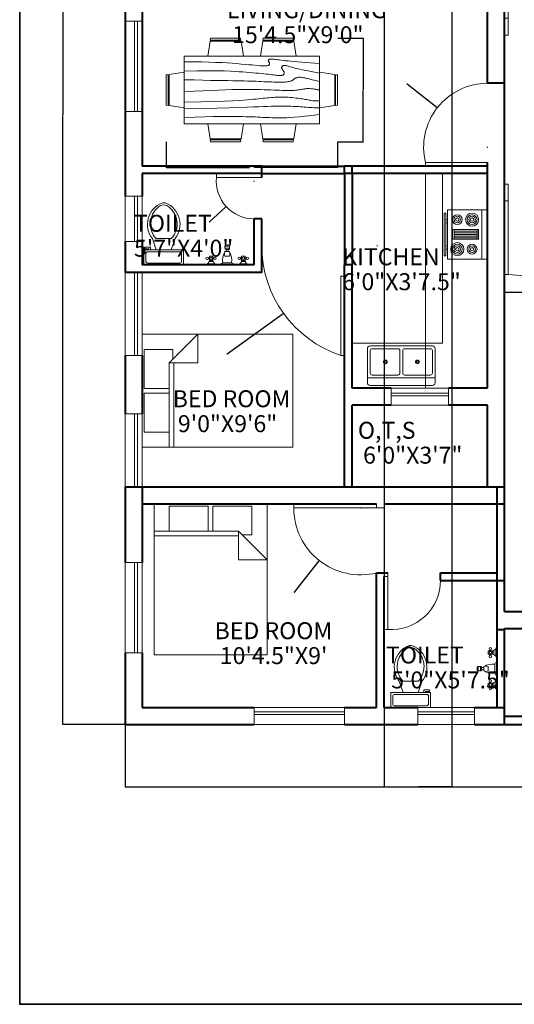
# Model space of a CAD drawing. Units: inches. Extents: x 2220 to 3422, y 783 to 1748.
# Tile 1 of 7: x 2220 to 2483, y 783 to 1306. Entities that reach past the tile are written whole.
import ezdxf

# ---------------------------------------------------------------- set-up
doc = ezdxf.new("R2010")
doc.units = ezdxf.units.IN
for name, color, linetype, lineweight in [('A-ANNO-DIMS', 2, 'Continuous', 18), ('A-ANNO-TTLB', 7, 'Continuous', 35), ('A-AREA-IDEN', 7, 'Continuous', 18), ('A-DOOR', 3, 'Continuous', 20), ('A-EQPM', 9, 'Continuous', 18), ('A-FLOR-CASE', 8, 'Continuous', 18), ('A-FLOR-FIXT', 9, 'Continuous', 18), ('A-FURN', 8, 'Continuous', 18), ('A-GLAZ', 4, 'Continuous', 18), ('A-WALL', 7, 'Continuous', 40)]:
    doc.layers.add(name, color=color, linetype=linetype, lineweight=lineweight)
doc.styles.get("Standard").update_dxf_attribs({"font": 'arial.ttf'})
doc.dimstyles.get("Standard").update_dxf_attribs({"dimtxt": 0.18, "dimasz": 0.18, "dimexe": 0.18, "dimexo": 0.0625, "dimgap": 0.09, "dimtad": 0, "dimtih": 1, "dimtoh": 1, "dimdec": 4, "dimzin": 0, "dimdsep": 46, "dimtxsty": 'Standard', "dimcen": 0.09, "dimadec": 0, "dimazin": 0, "dimtfac": 1, "dimtdec": 4, "dimtofl": 0, "dimtmove": 0, "dimatfit": 3, "dimfxl": 1, "dimtolj": 1, "dimtzin": 0, "dimarcsym": 0})

# ---------------------------------------------------------------- blocks, each defined once
blk = doc.blocks.new('Toilet - top')
for p, q in [((9.5, -6), (9.5, -2)), ((-10, -8.5), (-8, -8.5)), ((-10, -9.5), (-10, -8.5)), ((-7, -9.5), (-10, -9.5)), ((-8, -8.5), (-8, -8)), ((-7, -8), (-7, -9.5)), ((-4, -8), (-6, -14)), ((4, -8), (6, -14)), ((4, -14), (-4, -14))]:
    blk.add_line(p, q)
blk.add_lwpolyline([(10.5, -8), (10.5, 0), (-10.5, 0), (-10.5, -8)], close=True)
for points in [[(-9.5, -2), (-9.5, -6)], [(8.5, -1), (-8.5, -1)], [(-8.5, -7), (8.5, -7)]]:
    blk.add_lwpolyline(points)
for centre, radius, start, end in [((-8.62, -1.88), 0.884, 81.8699, 188.1301), ((8.62, -1.88), 0.884, 351.8699, 98.1301), ((-8.62, -6.12), 0.884, 171.8699, 278.1301), ((8.62, -6.12), 0.884, 261.8699, 8.1301), ((3.52, -21.58), 12.17, 141.4691, 247.9714), ((4.2, -21.82), 11.33, 136.3677, 238.9468), ((-3.52, -21.58), 12.17, 292.0284, 38.5307), ((-4.2, -21.82), 11.33, 301.053, 43.6321), ((0, -27.88), 4, 245.7318, 294.2682), ((0, -29), 4, 254.8605, 285.1395)]:
    blk.add_arc(centre, radius, start, end)
blk = doc.blocks.new('Faucet - Bathroom front')
for p, q in [((-0.5, 4.25), (0.5, 4.25)), ((0.5, 3.75), (-0.5, 3.75)), ((-0.5, 3), (0.5, 3)), ((-0.25, 3), (-0.25, 3.5)), ((0.25, 3.5), (0.25, 3)), ((-5, 0), (-2.25, 0)), ((-4.5087, 0.25), (-2.7408, 0.25)), ((-4, 1.625), (-4.25, 1.625)), ((-4, 1.375), (-4.25, 1.375)), ((-3.1442, 0.75), (-4.0979, 0.75)), ((-3.25, 1.625), (-3, 1.625)), ((-3.25, 1.375), (-3, 1.375)), ((-1.5, 0), (1.5, 0)), ((-1, 0.5), (1, 0.5)), ((0.5, 2), (-0.5, 2)), ((2.25, 0), (5, 0)), ((2.7413, 0.25), (4.5092, 0.25)), ((3.25, 1.625), (3, 1.625)), ((3.25, 1.375), (3, 1.375)), ((4.1058, 0.75), (3.1521, 0.75)), ((4, 1.625), (4.25, 1.625)), ((4, 1.375), (4.25, 1.375))]:
    blk.add_line(p, q)
for points in [[(-0.25, 4.5), (0.25, 4.5)], [(-0.5, 3.75), (-0.5, 4.25)], [(0.25, 3.5), (-0.25, 3.5)], [(0.5, 4.25), (0.5, 3.75)]]:
    blk.add_lwpolyline(points)
for points in [[(-4, 1), (-4, 2), (-3.25, 2), (-3.25, 1)], [(3.25, 1), (3.25, 2), (4, 2), (4, 1)]]:
    blk.add_lwpolyline(points, close=True)
for centre in [(-4.5, 1.5), (-3.625, 1.5), (-2.75, 1.5), (2.75, 1.5), (3.625, 1.5), (4.5, 1.5)]:
    blk.add_circle(centre, 0.2795)
for centre, radius, start, end in [((-0.2575, 4.2575), 0.2426, 88.22243, 181.7776), ((0.2575, 4.2575), 0.2426, 358.2224, 91.77757), ((3, 1), 4.0311, 150.2551, 187.125), ((0.6413, 2.5), 1.246, 156.3417, 203.6583), ((-0.2575, 3.7425), 0.2426, 178.2224, 271.7776), ((0.2575, 3.7425), 0.2426, 268.2224, 1.777565), ((-3, 1), 4.0311, 352.875, 29.74488), ((-0.6413, 2.5), 1.246, 336.3417, 23.65835), ((-5.375, 1.375), 1.4252, 285.2551, 344.7449), ((-1.875, 1.375), 1.4252, 195.2551, 254.7449), ((-0.7962, -0.2038), 0.7327, 106.1502, 163.8498), ((0.7962, -0.2038), 0.7327, 16.1502, 73.84979), ((1.875, 1.375), 1.4252, 285.2551, 344.7449), ((5.375, 1.375), 1.4252, 195.2551, 254.7449)]:
    blk.add_arc(centre, radius, start, end)
blk = doc.blocks.new('Range-Oven - 30 in top')
for p, q in [((0, -3), (30, -3)), ((12, -6), (18, -6)), ((13, -20), (13, -6)), ((14, -6), (14, -20)), ((15, -20), (15, -6)), ((16, -6), (16, -20)), ((17, -20), (17, -6)), ((18, -20), (12, -20)), ((6, -24), (6, -25)), ((8, -25), (8, -24)), ((22, -25), (22, -24)), ((24, -24), (24, -25))]:
    blk.add_line(p, q)
for points in [[(0, -24), (0, 0), (30, 0), (30, -24)], [(12, -21), (12, -5), (18, -5), (18, -21)], [(2, -26), (2, -25), (28, -25), (28, -26)]]:
    blk.add_lwpolyline(points, close=True)
for centre, radius in [((6, -9), 4), ((6, -9), 3), ((6, -9), 2), ((6, -9), 1), ((24, -9), 3), ((24, -9), 2), ((24, -9), 1), ((6, -18), 3), ((6, -18), 2), ((6, -18), 1), ((24, -18), 4), ((24, -18), 3), ((24, -18), 2), ((24, -18), 1)]:
    blk.add_circle(centre, radius)
blk = doc.blocks.new('Sink-double - 36 in top')
for p, q in [((-18, -4), (18, -4)), ((-0.75, -18.5), (-0.75, -6.5)), ((0.75, -6.5), (0.75, -18.5))]:
    blk.add_line(p, q)
for points in [[(-16.5, 0), (16.5, 0)], [(-18, -19.5), (-18, -1.5)], [(18, -1.5), (18, -19.5)], [(-16.5, -18.5), (-16.5, -6.5)], [(-15.5, -5.5), (-1.75, -5.5)], [(1.75, -5.5), (15.5, -5.5)], [(16.5, -6.5), (16.5, -18.5)], [(-1.75, -19.5), (-15.5, -19.5)], [(15.5, -19.5), (1.75, -19.5)], [(16.5, -21), (-16.5, -21)]]:
    blk.add_lwpolyline(points)
for centre, radius in [((-8.5, -12.5), 1), ((-8.5, -12.5), 0.5), ((8.5, -12.5), 1), ((8.5, -12.5), 0.5)]:
    blk.add_circle(centre, radius)
for centre, radius, start, end in [((-16.5, -1.5), 1.5, 90, 180), ((16.5, -1.5), 1.5, 0, 90), ((-15.5, -6.5), 1, 90, 180), ((-1.75, -6.5), 1, 0, 90), ((1.75, -6.5), 1, 90, 180), ((15.5, -6.5), 1, 0, 90), ((-16.5, -19.5), 1.5, 180, 270), ((-15.5, -18.5), 1, 180, 270), ((-1.75, -18.5), 1, 270, 0), ((1.75, -18.5), 1, 180, 270), ((15.5, -18.5), 1, 270, 0), ((16.5, -19.5), 1.5, 270, 0)]:
    blk.add_arc(centre, radius, start, end)
blk = doc.blocks.new('Bed - Queen')
for p, q in [((0, -80.00003), (0, 0)), ((0, 0), (59.99999, 0)), ((59.99999, 0), (59.99999, -80.00003)), ((7.99999, -1.2), (28.79998, -1.2)), ((7.99999, -14.4), (7.99999, -1.2)), ((28.79998, -1.2), (28.79998, -14.4)), ((31.19999, -1.2), (51.99999, -1.2)), ((31.19999, -14.4), (31.19999, -1.2)), ((51.99999, -1.2), (51.99999, -16.4)), ((0, -14.4), (44.8, -14.4)), ((59.99999, -29.6), (44.8, -14.4)), ((44.8, -14.4), (44.8, -29.6)), ((44.8, -16.8), (0, -16.8)), ((51.99999, -16.4), (46.79936, -16.4)), ((44.8, -29.6), (59.99999, -29.6)), ((59.99999, -80.00003), (0, -80.00003))]:
    blk.add_line(p, q)
blk = doc.blocks.new('Dining Set - 36 x 72 in.')
for p, q in [((-22, 27.5), (-22.1562, 26.50042)), ((-5.8416, 26.5), (-22.1534, 26.5)), ((-22, 27.5), (-6, 27.5)), ((-5.8437, 26.49966), (-6, 27.5)), ((6, 27.5), (5.8438, 26.50042)), ((22.1584, 26.5), (5.8466, 26.5)), ((6, 27.5), (22, 27.5)), ((22.1563, 26.49966), (22, 27.5)), ((-22.2343, 26.00059), (-23.4847, 17.99762)), ((-22.2304, 26), (-5.7608, 26)), ((-4.5152, 17.99762), (-5.7655, 25.99926)), ((5.7657, 26.00059), (4.5153, 17.99762)), ((5.7696, 26), (22.2392, 26)), ((23.4848, 17.99762), (22.2345, 25.99926)), ((36, 18), (-36, 18)), ((-36, 18), (-36, -18)), ((36, -18), (36, 18)), ((-45.5, 8), (-44.5004, 8.15617)), ((-45.5, 8), (-45.5, -8)), ((-44.5, -8.15843), (-44.5, 8.15338)), ((-44.0006, 8.23428), (-35.9976, 9.48474)), ((-44, 8.23041), (-44, -8.23915)), ((44.0006, 8.23428), (35.9976, 9.48474)), ((44, 8.23041), (44, -8.23915)), ((44.5, -8.15843), (44.5, 8.15338)), ((45.5, 8), (44.5005, 8.15617)), ((45.5, 8), (45.5, -8)), ((-44.4997, -8.15631), (-45.5, -8)), ((-35.9976, -9.48476), (-43.9993, -8.2345)), ((35.9976, -9.48476), (43.9993, -8.2345)), ((44.4997, -8.15631), (45.5, -8)), ((-36, -18), (36, -18)), ((-22.2343, -26.0006), (-23.4847, -17.99762)), ((-4.5152, -17.99762), (-5.7655, -25.99928)), ((5.7657, -26.0006), (4.5153, -17.99762)), ((23.4848, -17.99762), (22.2345, -25.99928)), ((-22.2304, -26), (-5.7608, -26)), ((5.7696, -26), (22.2392, -26)), ((-22, -27.5), (-22.1562, -26.50044)), ((-5.8416, -26.5), (-22.1534, -26.5)), ((-22, -27.5), (-6, -27.5)), ((-5.8437, -26.49967), (-6, -27.5)), ((6, -27.5), (5.8438, -26.50044)), ((22.1584, -26.5), (5.8466, -26.5)), ((6, -27.5), (22, -27.5)), ((22.1563, -26.49967), (22, -27.5))]:
    blk.add_line(p, q)
for points in [[(-36, 15), (-31.1772, 14.97754), (-26.8079, 14.91406), (-22.8538, 14.81543), (-19.276, 14.6875), (-16.0362, 14.53613), (-13.0957, 14.36718), (-10.4159, 14.18652), (-7.9583, 14), (-5.6904, 13.81315), (-3.6035, 13.63021), (-1.6954, 13.45508), (0.0365, 13.29166), (1.5945, 13.14388), (2.9811, 13.01562), (4.1988, 12.9108), (5.25, 12.83333), (6.1393, 12.78613), (6.8802, 12.76823), (7.4883, 12.77767), (7.9792, 12.8125), (8.3685, 12.87077), (8.6719, 12.95052), (8.9049, 13.0498), (9.0833, 13.16666), (9.2205, 13.29899), (9.3216, 13.44401), (9.3895, 13.59879), (9.4271, 13.76041), (9.4373, 13.92594), (9.4232, 14.09245), (9.3875, 14.257), (9.3333, 14.41666), (9.2638, 14.56917), (9.1836, 14.71484), (9.0975, 14.85465), (9.0104, 14.98958), (8.9272, 15.1206), (8.8529, 15.2487), (8.7922, 15.37483), (8.75, 15.5), (8.7305, 15.62467), (8.7344, 15.74739), (8.7617, 15.86621), (8.8125, 15.97916), (8.8867, 16.08431), (8.9844, 16.17968), (9.1055, 16.26334), (9.25, 16.33333), (9.4189, 16.38802), (9.6172, 16.42708), (9.8506, 16.45052), (10.125, 16.45833), (10.4463, 16.45052), (10.8203, 16.42708), (11.2529, 16.38802), (11.75, 16.33333), (12.3184, 16.26318), (12.9694, 16.17838), (13.7151, 16.07991), (14.5677, 15.96875), (15.5395, 15.84586), (16.6426, 15.71224), (17.8893, 15.56884), (19.2917, 15.41666), (20.859, 15.25667), (22.5879, 15.08984), (24.4721, 14.91715), (26.5052, 14.73958), (28.6809, 14.5581), (30.9929, 14.3737), (33.4347, 14.18733), (36, 14)], [(-36, 10), (-28.9766, 10.14274), (-23.1725, 10.20442), (-18.4241, 10.19775), (-14.5677, 10.13541), (-11.4399, 10.03011), (-8.877, 9.89453), (-6.7154, 9.74137), (-4.7917, 9.58333), (-2.9698, 9.43082), (-1.2246, 9.28515), (0.4415, 9.14534), (2.026, 9.01041), (3.5266, 8.87939), (4.9408, 8.7513), (6.266, 8.62516), (7.5, 8.5), (8.6411, 8.37549), (9.6914, 8.2539), (10.6538, 8.13818), (11.5312, 8.03125), (12.3267, 7.93603), (13.043, 7.85547), (13.6831, 7.79248), (14.25, 7.75), (14.7471, 7.7303), (15.1797, 7.73307), (15.5537, 7.75732), (15.875, 7.80208), (16.1494, 7.86637), (16.3828, 7.94922), (16.5811, 8.04964), (16.75, 8.16666), (16.8944, 8.29915), (17.0143, 8.44531), (17.1089, 8.60319), (17.1771, 8.77083), (17.218, 8.94629), (17.2305, 9.1276), (17.2137, 9.31282), (17.1667, 9.5), (17.0895, 9.6875), (16.987, 9.875), (16.8649, 10.0625), (16.7292, 10.25), (16.5856, 10.4375), (16.4401, 10.625), (16.2985, 10.8125), (16.1667, 11), (16.05, 11.18733), (15.9518, 11.3737), (15.8752, 11.5581), (15.8229, 11.73958), (15.798, 11.91715), (15.8034, 12.08984), (15.842, 12.25667), (15.9167, 12.41666), (16.0295, 12.56836), (16.1784, 12.70833), (16.3605, 12.83268), (16.5729, 12.9375), (16.8127, 13.01888), (17.0768, 13.07291), (17.3625, 13.0957), (17.6667, 13.08333), (17.9894, 13.03312), (18.3418, 12.94726), (18.7382, 12.82918), (19.1927, 12.68229), (19.7195, 12.51001), (20.3327, 12.31575), (21.0465, 12.10294), (21.875, 11.875), (22.8357, 11.63354), (23.959, 11.37304), (25.2786, 11.08618), (26.8282, 10.76562), (28.6414, 10.40405), (30.752, 9.99414), (33.1936, 9.52856), (36, 9)], [(-36, 5.5), (-30.7157, 5.3348), (-26.069, 5.20963), (-21.9946, 5.11767), (-18.4271, 5.05208), (-15.3009, 5.00602), (-12.5508, 4.97265), (-10.1112, 4.94515), (-7.9167, 4.91666), (-5.909, 4.88167), (-4.0586, 4.83984), (-2.3429, 4.79215), (-0.7396, 4.73958), (0.7739, 4.6831), (2.22, 4.6237), (3.6213, 4.56233), (5, 4.5), (6.373, 4.43782), (7.7344, 4.3776), (9.0723, 4.32129), (10.375, 4.27083), (11.6309, 4.22819), (12.8281, 4.19531), (13.9551, 4.17415), (15, 4.16666), (15.954, 4.17448), (16.819, 4.19791), (17.6001, 4.23698), (18.3021, 4.29166), (18.9299, 4.36198), (19.4883, 4.44791), (19.9823, 4.54948), (20.4167, 4.66666), (20.7969, 4.79899), (21.1302, 4.94401), (21.4245, 5.09879), (21.6875, 5.26041), (21.9271, 5.42594), (22.1511, 5.59245), (22.3672, 5.757), (22.5834, 5.91666), (22.8065, 6.06868), (23.0404, 6.21093), (23.2879, 6.34147), (23.5521, 6.45833), (23.8358, 6.55957), (24.142, 6.64323), (24.4735, 6.70735), (24.8334, 6.75), (25.2235, 6.76969), (25.642, 6.76692), (26.0858, 6.74267), (26.5521, 6.69791), (27.0379, 6.63362), (27.5404, 6.55078), (28.0565, 6.45036), (28.5834, 6.33333), (29.1242, 6.19987), (29.7071, 6.04687), (30.3661, 5.87044), (31.1354, 5.66666), (32.0493, 5.43164), (33.142, 5.16146), (34.4475, 4.85221), (36, 4.5)], [(-36, -1), (-30.7915, -0.6591), (-26.0195, -0.38216), (-21.6519, -0.16284), (-17.6563, 0.00521), (-14.0005, 0.12833), (-10.6523, 0.21289), (-7.5796, 0.26522), (-4.75, 0.29166), (-2.134, 0.29793), (0.2878, 0.28711), (2.5317, 0.26163), (4.6146, 0.22396), (6.5529, 0.17651), (8.3633, 0.12174), (10.0623, 0.06209), (11.6667, 0), (13.1899, -0.06201), (14.6341, -0.1211), (15.9982, -0.17432), (17.2813, -0.21875), (18.4823, -0.25147), (19.6003, -0.26953), (20.6343, -0.27002), (21.5834, -0.25), (22.4481, -0.20768), (23.2357, -0.14584), (23.9549, -0.06836), (24.6146, 0.02083), (25.2235, 0.11784), (25.7904, 0.21875), (26.3241, 0.31966), (26.8334, 0.41666), (27.3265, 0.50618), (27.8099, 0.58593), (28.2894, 0.65397), (28.7709, 0.70833), (29.2601, 0.74707), (29.763, 0.76823), (30.2855, 0.76985), (30.8334, 0.75), (31.4088, 0.70784), (31.9994, 0.64713), (32.589, 0.57275), (33.1615, 0.48958), (33.7008, 0.4025), (34.1908, 0.3164), (34.6153, 0.23616), (34.9584, 0.16666), (35.2099, 0.11165), (35.3848, 0.07031), (35.504, 0.04069), (35.5886, 0.02083), (35.6594, 0.00879), (35.7377, 0.0026), (35.8442, 0.00032), (36, 0)], [(-36, -6.5), (-27.1843, -6.31267), (-20.084, -6.1263), (-14.469, -5.9419), (-10.1094, -5.76042), (-6.7752, -5.58285), (-4.2363, -5.41016), (-2.2629, -5.24333), (-0.625, -5.08334), (0.8708, -4.93099), (2.2715, -4.78646), (3.5872, -4.64974), (4.8281, -4.52084), (6.0046, -4.39974), (7.127, -4.28646), (8.2053, -4.18099), (9.25, -4.08334), (10.2705, -3.99382), (11.2734, -3.91407), (12.2647, -3.84603), (13.25, -3.79167), (14.2354, -3.75293), (15.2266, -3.73177), (16.2295, -3.73015), (17.25, -3.75), (18.2912, -3.79248), (19.3451, -3.85547), (20.4009, -3.93604), (21.4479, -4.03125), (22.4754, -4.13819), (23.4727, -4.25391), (24.4289, -4.37549), (25.3334, -4.5), (26.1785, -4.62492), (26.9694, -4.74935), (27.7145, -4.87281), (28.4219, -4.99479), (29.1, -5.11483), (29.7572, -5.23242), (30.4016, -5.34709), (31.0417, -5.45834), (31.6837, -5.56437), (32.3262, -5.65821), (32.9658, -5.73153), (33.599, -5.77604), (34.2224, -5.78345), (34.8327, -5.74545), (35.4264, -5.65373), (36, -5.5)], [(-36, -10), (-26.4022, -9.81299), (-18.4675, -9.62891), (-11.9839, -9.45069), (-6.7396, -9.28125), (-2.5226, -9.12354), (0.8789, -8.98047), (3.6769, -8.85498), (6.0833, -8.75), (8.2767, -8.66765), (10.3021, -8.60677), (12.1712, -8.56543), (13.8958, -8.54167), (15.4876, -8.53353), (16.9583, -8.53907), (18.3197, -8.55632), (19.5834, -8.58334), (20.7616, -8.61841), (21.8685, -8.66081), (22.9188, -8.71004), (23.9271, -8.76563), (24.9081, -8.82707), (25.8763, -8.89388), (26.8465, -8.96558), (27.8334, -9.04167), (28.8474, -9.12118), (29.8828, -9.20117), (30.93, -9.27824), (31.9792, -9.34896), (33.0205, -9.40991), (34.0443, -9.45768), (35.0407, -9.48885), (36, -9.5)], [(-36, -14.5), (-30.0881, -14.33513), (-25.0332, -14.21224), (-20.7312, -14.12647), (-17.0781, -14.07292), (-13.97, -14.04671), (-11.3027, -14.04297), (-8.9724, -14.05681), (-6.875, -14.08334), (-4.9224, -14.11833), (-3.0905, -14.16016), (-1.3709, -14.20785), (0.2448, -14.26042), (1.7647, -14.3169), (3.1973, -14.3763), (4.5507, -14.43767), (5.8333, -14.5), (7.0554, -14.5621), (8.235, -14.62175), (9.3922, -14.67652), (10.5469, -14.72396), (11.7192, -14.76164), (12.929, -14.78711), (14.1965, -14.79794), (15.5417, -14.79167), (16.9933, -14.76424), (18.6152, -14.70508), (20.4804, -14.60197), (22.6615, -14.44271), (25.2312, -14.21509), (28.2624, -13.9069), (31.8277, -13.50594), (36, -13)]]:
    blk.add_lwpolyline(points)
blk = doc.blocks.new('DOOR-UNIT-ENTRY')
for p, q in [((0, 48.53), (2, 48.53)), ((2, 0.53), (2, 48.53)), ((48, 39.53), (48, 48.53)), ((0, 39.53), (2, 39.53)), ((0, 0.53), (2, 0.53))]:
    blk.add_line(p, q)
blk.add_arc((8.47, 39.53), 39.53, 260.5843, 0)
blk = doc.blocks.new('WIN-48-OFFSET-A')
for p, q in [((0, 0), (0, 9)), ((0, 9), (48, 9)), ((0, 6.75), (48, 6.75)), ((0, 5.25), (48, 5.25)), ((48, 0), (48, 9)), ((0, 0), (48, 0))]:
    blk.add_line(p, q)
blk = doc.blocks.new('WIN-48-OFFSET-B')
for p, q in [((0, 48), (9, 48)), ((0, 48), (0, 0)), ((5, 48), (5, 0)), ((6.5, 48), (6.5, 0)), ((9, 48), (9, 0)), ((0, 0), (9, 0))]:
    blk.add_line(p, q)
blk = doc.blocks.new('*D31')
at = {"layer": 'A-ANNO-DIMS', "color": 0, "lineweight": -2, "transparency": 16777216}
for p, q in [((2297.84, 1240.73), (2297.84, 1226.96)), ((2388.84, 1240.73), (2388.84, 1226.96)), ((2298.02, 1227.14), (2342.06, 1227.14)), ((2388.66, 1227.14), (2344.62, 1227.14))]:
    blk.add_line(p, q, dxfattribs=at)
at = {"layer": 'A-ANNO-DIMS', "color": 0, "transparency": 16777216}
for points in [[(2298.02, 1227.17), (2298.02, 1227.11), (2297.84, 1227.14)], [(2388.66, 1227.17), (2388.66, 1227.11), (2388.84, 1227.14)]]:
    blk.add_solid(points, dxfattribs=at)
at = {"layer": 'Defpoints', "color": 0, "transparency": 16777216}
for p in [(2297.84, 1240.79), (2388.84, 1240.79), (2388.84, 1227.14)]:
    blk.add_point(p, dxfattribs=at)
at = {"layer": 'A-ANNO-DIMS', "color": 0, "transparency": 16777216, "insert": (2343.34, 1227.14), "char_height": 0.18, "attachment_point": 5}
blk.add_mtext('\\A1;DINING SET 91 TYP.', dxfattribs=at)
blk = doc.blocks.new('*D32')
at = {"layer": 'A-ANNO-DIMS', "color": 0, "lineweight": -2, "transparency": 16777216}
for p, q in [((2388.91, 1295.79), (2402.67, 1295.79)), ((2402.49, 1295.61), (2402.49, 1268.47)), ((2402.49, 1240.97), (2402.49, 1268.11)), ((2388.91, 1240.79), (2402.67, 1240.79))]:
    blk.add_line(p, q, dxfattribs=at)
at = {"layer": 'A-ANNO-DIMS', "color": 0, "transparency": 16777216}
for points in [[(2402.46, 1295.61), (2402.52, 1295.61), (2402.49, 1295.79)], [(2402.46, 1240.97), (2402.52, 1240.97), (2402.49, 1240.79)]]:
    blk.add_solid(points, dxfattribs=at)
at = {"layer": 'Defpoints', "color": 0, "transparency": 16777216}
for p in [(2388.84, 1295.79), (2402.49, 1295.79), (2388.84, 1240.79)]:
    blk.add_point(p, dxfattribs=at)
at = {"layer": 'A-ANNO-DIMS', "color": 0, "transparency": 16777216, "insert": (2402.49, 1268.29), "char_height": 0.18, "attachment_point": 5}
blk.add_mtext('\\A1;55 TYP.', dxfattribs=at)
blk = doc.blocks.new('*D40')
at = {"layer": 'A-ANNO-DIMS', "color": 0, "lineweight": -2, "transparency": 16777216}
for p, q in [((2477.55, 1168.43), (2477.55, 1160.83)), ((2525.55, 1168.43), (2525.55, 1160.83)), ((2477.73, 1161.01), (2501.01, 1161.01)), ((2525.37, 1161.01), (2502.08, 1161.01))]:
    blk.add_line(p, q, dxfattribs=at)
at = {"layer": 'A-ANNO-DIMS', "color": 0, "transparency": 16777216}
for points in [[(2477.73, 1161.04), (2477.73, 1160.98), (2477.55, 1161.01)], [(2525.37, 1161.04), (2525.37, 1160.98), (2525.55, 1161.01)]]:
    blk.add_solid(points, dxfattribs=at)
at = {"layer": 'Defpoints', "color": 0, "transparency": 16777216}
for p in [(2477.55, 1168.49), (2525.55, 1168.49), (2525.55, 1161.01)]:
    blk.add_point(p, dxfattribs=at)
at = {"layer": 'A-ANNO-DIMS', "color": 0, "transparency": 16777216, "insert": (2501.55, 1161.01), "char_height": 0.18, "attachment_point": 5}
blk.add_mtext('\\A1;48 TYP.', dxfattribs=at)
blk = doc.blocks.new('*D53')
at = {"layer": 'A-ANNO-DIMS', "color": 0, "lineweight": -2, "transparency": 16777216}
for p, q in [((2276.05, 931.33), (2276.05, 898.06)), ((2706.55, 931.33), (2706.55, 898.06)), ((2276.23, 898.24), (2490.9, 898.24)), ((2706.37, 898.24), (2491.69, 898.24))]:
    blk.add_line(p, q, dxfattribs=at)
at = {"layer": 'A-ANNO-DIMS', "color": 0, "transparency": 16777216}
for points in [[(2276.23, 898.27), (2276.23, 898.21), (2276.05, 898.24)], [(2706.37, 898.27), (2706.37, 898.21), (2706.55, 898.24)]]:
    blk.add_solid(points, dxfattribs=at)
at = {"layer": 'Defpoints', "color": 0, "transparency": 16777216}
for p in [(2276.05, 931.39), (2706.55, 931.39), (2706.55, 898.24)]:
    blk.add_point(p, dxfattribs=at)
at = {"layer": 'A-ANNO-DIMS', "color": 0, "transparency": 16777216, "insert": (2491.3, 898.24), "char_height": 0.18, "attachment_point": 5}
blk.add_mtext('\\A1;430.5', dxfattribs=at)
blk = doc.blocks.new('*D54')
at = {"layer": 'A-ANNO-DIMS', "color": 0, "lineweight": -2, "transparency": 16777216}
for p, q in [((2275.98, 1578.39), (2242.72, 1578.39)), ((2242.9, 1578.21), (2242.9, 1255.07)), ((2242.9, 931.57), (2242.9, 1254.71)), ((2275.98, 931.39), (2242.72, 931.39))]:
    blk.add_line(p, q, dxfattribs=at)
at = {"layer": 'A-ANNO-DIMS', "color": 0, "transparency": 16777216}
for points in [[(2242.87, 1578.21), (2242.93, 1578.21), (2242.9, 1578.39)], [(2242.87, 931.57), (2242.93, 931.57), (2242.9, 931.39)]]:
    blk.add_solid(points, dxfattribs=at)
at = {"layer": 'Defpoints', "color": 0, "transparency": 16777216}
for p in [(2242.9, 1578.39), (2276.05, 1578.39), (2276.05, 931.39)]:
    blk.add_point(p, dxfattribs=at)
at = {"layer": 'A-ANNO-DIMS', "color": 0, "transparency": 16777216, "insert": (2242.9, 1254.89), "char_height": 0.18, "attachment_point": 5}
blk.add_mtext('\\A1;647', dxfattribs=at)
blk = doc.blocks.new('*D73')
at = {"layer": 'A-ANNO-DIMS', "color": 0, "lineweight": -2, "transparency": 16777216}
for p, q in [((2413.55, 1501.83), (2413.55, 898.06)), ((2449.55, 1501.83), (2449.55, 898.06)), ((2413.73, 898.24), (2431.33, 898.24)), ((2449.37, 898.24), (2431.77, 898.24))]:
    blk.add_line(p, q, dxfattribs=at)
at = {"layer": 'A-ANNO-DIMS', "color": 0, "transparency": 16777216}
for points in [[(2413.73, 898.27), (2413.73, 898.21), (2413.55, 898.24)], [(2449.37, 898.27), (2449.37, 898.21), (2449.55, 898.24)]]:
    blk.add_solid(points, dxfattribs=at)
at = {"layer": 'Defpoints', "color": 0, "transparency": 16777216}
for p in [(2413.55, 1501.89), (2449.55, 1501.89), (2449.55, 898.24)]:
    blk.add_point(p, dxfattribs=at)
at = {"layer": 'A-ANNO-DIMS', "color": 0, "transparency": 16777216, "insert": (2431.55, 898.24), "char_height": 0.18, "attachment_point": 5}
blk.add_mtext('\\A1;36', dxfattribs=at)
blk = doc.blocks.new('*D74')
at = {"layer": 'A-ANNO-DIMS', "color": 0, "lineweight": -2, "transparency": 16777216}
for p, q in [((2409.85, 1185.64), (2410.03, 1185.64)), ((2409.94, 1185.55), (2409.94, 1185.73)), ((2330.26, 1128.19), (2360, 1149.63)), ((2330.08, 1128.19), (2330.26, 1128.19))]:
    blk.add_line(p, q, dxfattribs=at)
at = {"layer": 'A-ANNO-DIMS', "color": 0, "transparency": 16777216}
blk.add_solid([(2359.98, 1149.65), (2360.01, 1149.6), (2360.14, 1149.73)], dxfattribs=at)
at = {"layer": 'Defpoints', "color": 0, "transparency": 16777216}
for p in [(2409.94, 1185.64), (2360.14, 1149.73)]:
    blk.add_point(p, dxfattribs=at)
at = {"layer": 'A-ANNO-DIMS', "color": 0, "transparency": 16777216, "insert": (2329.6, 1128.19), "char_height": 0.18, "attachment_point": 5}
blk.add_mtext('\\A1;R61.39', dxfattribs=at)
blk = doc.blocks.new('*D80')
at = {"layer": 'A-ANNO-DIMS', "color": 0, "lineweight": -2, "transparency": 16777216}
for p, q in [((2400.98, 1046.39), (2401.16, 1046.39)), ((2401.07, 1046.3), (2401.07, 1046.48)), ((2366, 1001.66), (2379.04, 1018.29)), ((2365.82, 1001.66), (2366, 1001.66))]:
    blk.add_line(p, q, dxfattribs=at)
at = {"layer": 'A-ANNO-DIMS', "color": 0, "transparency": 16777216}
blk.add_solid([(2379.02, 1018.31), (2379.06, 1018.27), (2379.15, 1018.43)], dxfattribs=at)
at = {"layer": 'Defpoints', "color": 0, "transparency": 16777216}
for p in [(2401.07, 1046.39), (2379.15, 1018.43)]:
    blk.add_point(p, dxfattribs=at)
at = {"layer": 'A-ANNO-DIMS', "color": 0, "transparency": 16777216, "insert": (2365.27, 1001.66), "char_height": 0.18, "attachment_point": 5}
blk.add_mtext('\\A1;R35.526', dxfattribs=at)
blk = doc.blocks.new('*D81')
at = {"layer": 'A-ANNO-DIMS', "color": 0, "lineweight": -2, "transparency": 16777216}
for p, q in [((2425.64, 1271.5), (2425.82, 1271.5)), ((2425.82, 1271.5), (2441.7, 1259.02)), ((2468.46, 1237.93), (2468.64, 1237.93)), ((2468.55, 1237.84), (2468.55, 1238.02))]:
    blk.add_line(p, q, dxfattribs=at)
at = {"layer": 'A-ANNO-DIMS', "color": 0, "transparency": 16777216}
blk.add_solid([(2441.72, 1259.04), (2441.68, 1259), (2441.84, 1258.91)], dxfattribs=at)
at = {"layer": 'Defpoints', "color": 0, "transparency": 16777216}
for p in [(2441.84, 1258.91), (2468.55, 1237.93)]:
    blk.add_point(p, dxfattribs=at)
at = {"layer": 'A-ANNO-DIMS', "color": 0, "transparency": 16777216, "insert": (2425.09, 1271.5), "char_height": 0.18, "attachment_point": 5}
blk.add_mtext('\\A1;R33.964', dxfattribs=at)
blk = doc.blocks.new('*D87')
at = {"layer": 'A-ANNO-DIMS', "color": 0, "lineweight": -2, "transparency": 16777216}
for p, q in [((2344.46, 1219.98), (2344.64, 1219.98)), ((2344.55, 1219.89), (2344.55, 1220.07)), ((2320.76, 1198.36), (2329.55, 1206.35)), ((2320.58, 1198.36), (2320.76, 1198.36))]:
    blk.add_line(p, q, dxfattribs=at)
at = {"layer": 'A-ANNO-DIMS', "color": 0, "transparency": 16777216}
blk.add_solid([(2329.53, 1206.37), (2329.57, 1206.32), (2329.68, 1206.47)], dxfattribs=at)
at = {"layer": 'Defpoints', "color": 0, "transparency": 16777216}
for p in [(2344.55, 1219.98), (2329.68, 1206.47)]:
    blk.add_point(p, dxfattribs=at)
at = {"layer": 'A-ANNO-DIMS', "color": 0, "transparency": 16777216, "insert": (2320.1, 1198.36), "char_height": 0.18, "attachment_point": 5}
blk.add_mtext('\\A1;R20.09', dxfattribs=at)

msp = doc.modelspace()

# ---------------------------------------------------------------- linework, layer by layer
at = {"layer": 'A-ANNO-TTLB'}
msp.add_lwpolyline([(2220.0037, 1747.9465), (3422.343, 1747.9465), (3422.343, 782.804), (2220.0037, 782.804)], close=True, dxfattribs=at)
at = {"layer": 'A-DOOR'}
for p, q in [((2479.5466, 1297.3907), (2477.5466, 1297.3907)), ((2468.5466, 1229.8907), (2435.5466, 1229.8907)), ((2435.5466, 1227.8907), (2435.5466, 1229.8907)), ((2324.5466, 1221.8907), (2324.5466, 1223.8907)), ((2348.5466, 1221.8907), (2324.5466, 1221.8907)), ((2392.5466, 1169.3907), (2390.5466, 1169.3907)), ((2390.5466, 1127.3907), (2390.5466, 1169.3907)), ((2392.5466, 1127.3907), (2390.5466, 1127.3907)), ((2365.5466, 1046.3907), (2365.5466, 1048.3907)), ((2413.5466, 1046.3907), (2365.5466, 1046.3907)), ((2409.5466, 1046.3907), (2409.5466, 1048.3907)), ((2413.5466, 1046.3907), (2413.5466, 1048.3907)), ((2413.5466, 1009.8907), (2415.5466, 1009.8907)), ((2415.5466, 981.8907), (2415.5466, 1011.8907)), ((2413.5466, 981.8907), (2415.5466, 981.8907))]:
    msp.add_line(p, q, dxfattribs=at)
for centre, radius, start, end in [((2468.5466, 1237.9264), 33.9643, 90, 193.685547), ((2344.5466, 1219.9816), 20.0909, 174.547378, 270), ((2409.9402, 1185.6407), 61.3936, 180, 251.585472), ((2401.0722, 1046.3907), 35.5256, 180, 283.800656), ((2417.4752, 1007.8907), 26.0714, 265.757807, 360)]:
    msp.add_arc(centre, radius, start, end, dxfattribs=at)
at = {"layer": 'A-FLOR-CASE'}
for p, q in [((2435.5466, 1109.8907), (2435.5466, 1223.8907)), ((2444.5466, 1133.8907), (2444.5466, 1223.8907)), ((2444.5466, 1133.8907), (2396.5466, 1133.8907))]:
    msp.add_line(p, q, dxfattribs=at)
at = {"layer": 'A-GLAZ'}
for p, q in [((2285.0466, 1304.8907), (2276.0466, 1304.8907)), ((2281.0466, 1304.8907), (2281.0466, 1256.8907)), ((2282.5466, 1304.8907), (2282.5466, 1256.8907)), ((2285.0466, 1256.8907), (2276.0466, 1256.8907)), ((2285.0466, 1211.8907), (2276.0466, 1211.8907)), ((2276.0466, 1211.8907), (2276.0466, 1187.8907)), ((2281.0466, 1211.8907), (2281.0466, 1187.8907)), ((2282.5466, 1211.8907), (2282.5466, 1187.8907)), ((2285.0466, 1211.8907), (2285.0466, 1187.8907)), ((2285.0466, 1187.8907), (2276.0466, 1187.8907)), ((2276.0466, 1171.3907), (2276.0466, 1127.3907)), ((2281.0466, 1171.3907), (2281.0466, 1127.3907)), ((2282.5466, 1171.3907), (2282.5466, 1127.3907)), ((2285.0466, 1171.3907), (2285.0466, 1127.3907)), ((2285.0466, 1127.3907), (2276.0466, 1127.3907)), ((2285.0466, 1127.3907), (2276.0466, 1127.3907)), ((2417.2966, 1100.8907), (2417.2966, 1109.8907)), ((2417.2966, 1109.8907), (2447.7966, 1109.8907)), ((2447.7966, 1100.8907), (2447.7966, 1109.8907)), ((2447.7966, 1107.3907), (2417.2966, 1107.3907)), ((2447.7966, 1105.8907), (2417.2966, 1105.8907)), ((2417.2966, 1100.8907), (2447.7966, 1100.8907)), ((2285.0466, 1096.3907), (2276.0466, 1096.3907)), ((2276.0466, 1096.3907), (2276.0466, 1057.3907)), ((2281.0466, 1096.3907), (2281.0466, 1057.3907)), ((2282.5466, 1096.3907), (2282.5466, 1057.3907)), ((2285.0466, 1096.3907), (2285.0466, 1057.3907)), ((2431.5466, 931.3907), (2431.5466, 940.3907)), ((2431.5466, 940.3907), (2461.5466, 940.3907)), ((2431.5466, 938.1407), (2461.5466, 938.1407)), ((2431.5466, 936.6407), (2461.5466, 936.6407)), ((2461.5466, 931.3907), (2461.5466, 940.3907)), ((2431.5466, 931.3907), (2461.5466, 931.3907))]:
    msp.add_line(p, q, dxfattribs=at)
at = {"layer": 'A-WALL'}
for p, q in [((2477.5466, 1109.8907), (2477.5466, 1461.3907)), ((2276.0466, 1362.6407), (2276.0466, 1211.8907)), ((2285.0466, 1335.8907), (2285.0466, 1227.8907)), ((2468.5466, 1271.8907), (2468.5466, 1335.8907)), ((2477.5466, 1271.8907), (2468.5466, 1271.8907)), ((2468.5466, 1109.8907), (2468.5466, 1229.8907)), ((2348.5466, 1227.8907), (2285.0466, 1227.8907)), ((2348.5466, 1223.8907), (2285.0466, 1223.8907)), ((2285.0466, 1223.8907), (2285.0466, 1211.8907)), ((2348.5466, 1221.8907), (2348.5466, 1227.8907)), ((2348.5466, 1227.8907), (2392.5466, 1227.8907)), ((2348.5466, 1223.8907), (2392.5466, 1223.8907)), ((2468.5466, 1227.8907), (2392.5466, 1227.8907)), ((2392.5466, 1223.8907), (2392.5466, 1227.8907)), ((2468.5466, 1223.8907), (2392.5466, 1223.8907)), ((2392.5466, 1223.8907), (2392.5466, 1175.3907)), ((2396.5466, 1223.8907), (2396.5466, 1227.8907)), ((2396.5466, 1223.8907), (2396.5466, 1175.3907)), ((2344.5466, 1175.3907), (2344.5466, 1199.8907)), ((2348.5466, 1199.8907), (2344.5466, 1199.8907)), ((2348.5466, 1171.3907), (2348.5466, 1199.8907)), ((2276.0466, 1187.8907), (2276.0466, 1171.3907)), ((2285.0466, 1187.8907), (2285.0466, 1175.3907)), ((2348.5466, 1171.3907), (2276.0466, 1171.3907)), ((2344.5466, 1175.3907), (2285.0466, 1175.3907)), ((2392.5466, 1109.8907), (2392.5466, 1175.3907)), ((2396.5466, 1175.3907), (2392.5466, 1175.3907)), ((2396.5466, 1109.8907), (2396.5466, 1175.3907)), ((2276.0466, 1127.3907), (2276.0466, 1096.3907)), ((2285.0466, 1127.3907), (2285.0466, 1096.3907)), ((2392.5466, 1057.3907), (2392.5466, 1109.8907)), ((2417.2966, 1109.8907), (2396.5466, 1109.8907)), ((2468.5466, 1109.8907), (2447.7966, 1109.8907)), ((2477.5466, 991.3907), (2477.5466, 1109.8907)), ((2396.5466, 1057.3907), (2396.5466, 1100.8907)), ((2417.2966, 1100.8907), (2396.5466, 1100.8907)), ((2468.5466, 1100.8907), (2447.7966, 1100.8907)), ((2468.5466, 1057.3907), (2468.5466, 1100.8907)), ((2477.5466, 1057.3907), (2276.0466, 1057.3907)), ((2276.0466, 1057.3907), (2276.0466, 1017.3907)), ((2285.0466, 1057.3907), (2285.0466, 1017.3907)), ((2473.5466, 940.3907), (2473.5466, 1057.3907)), ((2285.0466, 1048.3907), (2285.0466, 1017.3907)), ((2409.5466, 1048.3907), (2285.0466, 1048.3907)), ((2477.5466, 1048.3907), (2413.5466, 1048.3907)), ((2409.5466, 940.3907), (2409.5466, 1011.8907)), ((2409.5466, 1011.8907), (2415.5466, 1011.8907)), ((2413.5466, 940.3907), (2413.5466, 1009.8907)), ((2443.5466, 1007.8907), (2443.5466, 1011.8907)), ((2443.5466, 1011.8907), (2473.5466, 1011.8907)), ((2443.5466, 1007.8907), (2477.5466, 1007.8907)), ((2477.5466, 991.3907), (2488.5466, 991.3907)), ((2473.5466, 981.8907), (2477.5466, 981.8907)), ((2477.5466, 931.3907), (2477.5466, 982.3907)), ((2477.5466, 982.3907), (2488.5466, 982.3907)), ((2276.0466, 969.3907), (2276.0466, 931.3907)), ((2285.0466, 969.3907), (2285.0466, 940.3907)), ((2285.0466, 940.3907), (2344.5466, 940.3907)), ((2392.5466, 940.3907), (2409.5466, 940.3907)), ((2413.5466, 940.3907), (2431.5466, 940.3907)), ((2461.5466, 940.3907), (2477.5466, 940.3907)), ((2477.5466, 935.8907), (2585.5466, 935.8907)), ((2276.0466, 931.3907), (2344.5466, 931.3907)), ((2392.5466, 931.3907), (2431.5466, 931.3907)), ((2461.5466, 931.3907), (2477.5466, 931.3907)), ((2477.5466, 931.3907), (2585.5466, 931.3907))]:
    msp.add_line(p, q, dxfattribs=at)

# ---------------------------------------------------------------- block references
at = {"layer": 'A-DOOR', "extrusion": (0, 0, -1), "zscale": -1, "rotation": 180}
msp.add_blockref('DOOR-UNIT-ENTRY', (-2477.547, 1345.9234), dxfattribs=at)
at = {"layer": 'A-DOOR'}
msp.add_blockref('DOOR-UNIT-ENTRY', (2477.547, 1169.858), dxfattribs=at)
at = {"layer": 'A-EQPM', "xscale": 0.8722005701805317, "yscale": 0.8722005701805317, "zscale": 0.8722005701805317, "rotation": 270}
msp.add_blockref('Range-Oven - 30 in top', (2468.1505, 1204.7145), dxfattribs=at)
at = {"layer": 'A-FLOR-FIXT', "xscale": -1, "rotation": 180}
for name, p in [('Toilet - top', (2296.5234, 1175.4149)), ('Sink-double - 36 in top', (2422.697, 1111.4174))]:
    msp.add_blockref(name, p, dxfattribs=at)
at = {"layer": 'A-FLOR-FIXT', "yscale": 2.361580970438625, "zscale": 2.361580970438625}
for p, xscale, rotation in [((2330.2379, 1175.3907), -2.361580970438625, 359.9999999999942), ((2473.5466, 961.0174), 2.361580970438625, 90)]:
    msp.add_blockref('Faucet - Bathroom front', p, dxfattribs=dict(at, xscale=xscale, rotation=rotation))
at = {"layer": 'A-FLOR-FIXT', "rotation": 180}
msp.add_blockref('Toilet - top', (2427.6395, 940.3495), dxfattribs=at)
at = {"layer": 'A-FURN'}
for name, p in [('Dining Set - 36 x 72 in.', (2343.3428, 1268.2924)), ('Bed - Queen', (2291.3841, 1048.4524))]:
    msp.add_blockref(name, p, dxfattribs=at)
at = {"layer": 'A-FURN', "rotation": 90}
msp.add_blockref('Bed - Queen', (2285.0109, 1078.5691), dxfattribs=at)
at = {"layer": 'A-GLAZ'}
for name, p in [('WIN-48-OFFSET-B', (2276.047, 969.391)), ('WIN-48-OFFSET-A', (2344.547, 931.391))]:
    msp.add_blockref(name, p, dxfattribs=at)

# ---------------------------------------------------------------- texts
at = {"layer": 'A-AREA-IDEN'}
for s, p in [('LIVING/DINING', (2330.095, 1306.4078)), (' 15\'4.5"X9\'0"', (2330.095, 1293.1807)), ('TOILET', (2280.7264, 1193.0294)), ('5\'7"X4\'0"', (2280.7264, 1179.8023)), ('KITCHEN', (2391.312, 1175.225)), ('6\'0"X3\'7.5"', (2391.312, 1161.9979)), ('BED ROOM', (2301.2903, 1099.8624)), (' 9\'0"X9\'6"', (2301.2903, 1086.6354)), ('O,T,S', (2399.6524, 1083.1221)), (' 6\'0"X3\'7"', (2399.6524, 1069.895)), ('BED ROOM', (2323.5311, 976.696)), (' 10\'4.5"X9\'', (2323.5311, 963.469)), ('TOILET', (2414.5955, 963.788)), (' 5\'0"X5\'7.5"', (2414.5955, 950.561))]:
    msp.add_text(s, height=9, dxfattribs=at).set_placement(p)

# ---------------------------------------------------------------- dimensions: what is measured, and where the dimension line sits
at = {"layer": 'A-ANNO-DIMS'}
dim = msp.add_linear_dim(base=(2242.8966, 1578.3907), p1=(2276.0466, 931.3907), p2=(2276.0466, 1578.3907), angle=90, dimstyle='Standard', override={"dimdec": 0, "dimlfac": 1, "dimrnd": 0, "dimzin": 0, "dimdsep": 46, "dimlunit": 2}, dxfattribs=at)
dim.commit()
dim.dimension.update_dxf_attribs({"geometry": '*D54', "text_midpoint": (2242.8966, 1254.8907)})
for base, p1, p2, override, picture, middle in [((2449.5466, 898.2407), (2413.5466, 1501.8907), (2449.5466, 1501.8907), {"dimdec": 0, "dimlfac": 1, "dimrnd": 0, "dimzin": 0, "dimdsep": 46, "dimlunit": 2}, '*D73', (2431.5466, 898.2407)), ((2706.5466, 898.2407), (2276.0466, 931.3907), (2706.5466, 931.3907), {"dimdec": 1, "dimlfac": 1, "dimrnd": 0, "dimzin": 0, "dimdsep": 46, "dimlunit": 2}, '*D53', (2491.2966, 898.2407))]:
    dim = msp.add_linear_dim(base=base, p1=p1, p2=p2, dimstyle='Standard', override=override, dxfattribs=at)
    dim.commit()
    dim.dimension.update_dxf_attribs({"geometry": picture, "text_midpoint": middle})
dim = msp.add_linear_dim(base=(2402.4928, 1295.7924), p1=(2388.8428, 1240.7924), p2=(2388.8428, 1295.7924), angle=90, text='<> TYP.', dimstyle='Standard', override={"dimdec": 0, "dimlfac": 1, "dimrnd": 0, "dimzin": 0, "dimdsep": 46, "dimlunit": 2}, dxfattribs=at)
dim.commit()
dim.dimension.update_dxf_attribs({"geometry": '*D32', "text_midpoint": (2402.4928, 1268.2924)})
for center, mpoint, override, picture, middle in [((2468.5466, 1237.9264), (2441.8398, 1258.9102), {"dimdec": 3, "dimlfac": 1, "dimrnd": 0, "dimzin": 0, "dimdsep": 46, "dimlunit": 2}, '*D81', (2425.0863, 1271.5004)), ((2344.5466, 1219.9816), (2329.6808, 1206.4668), {"dimdec": 2, "dimlfac": 1, "dimrnd": 0, "dimzin": 0, "dimdsep": 46, "dimlunit": 2}, '*D87', (2320.1012, 1198.3579)), ((2409.9402, 1185.6407), (2360.1419, 1149.7339), {"dimdec": 2, "dimlfac": 1, "dimrnd": 0, "dimzin": 0, "dimdsep": 46, "dimlunit": 2}, '*D74', (2329.6028, 1128.1898)), ((2401.0722, 1046.3907), (2379.1521, 1018.4341), {"dimdec": 3, "dimlfac": 1, "dimrnd": 0, "dimzin": 0, "dimdsep": 46, "dimlunit": 2}, '*D80', (2365.2703, 1001.6601))]:
    dim = msp.add_radius_dim(center=center, mpoint=mpoint, dimstyle='Standard', override=override, dxfattribs=at)
    dim.commit()
    dim.dimension.update_dxf_attribs({"geometry": picture, "text_midpoint": middle, "dimtype": 164})
for base, p1, p2, text, picture, middle in [((2388.8428, 1227.1424), (2297.8428, 1240.7924), (2388.8428, 1240.7924), 'DINING SET <> TYP.', '*D31', (2343.3428, 1227.1424)), ((2525.5466, 1161.0055), (2477.5466, 1168.4905), (2525.5466, 1168.4905), '<> TYP.', '*D40', (2501.5466, 1161.0055))]:
    dim = msp.add_linear_dim(base=base, p1=p1, p2=p2, text=text, dimstyle='Standard', override={"dimdec": 0, "dimlfac": 1, "dimrnd": 0, "dimzin": 0, "dimdsep": 46, "dimlunit": 2}, dxfattribs=at)
    dim.commit()
    dim.dimension.update_dxf_attribs({"geometry": picture, "text_midpoint": middle})

doc.saveas('drawing.dxf')
